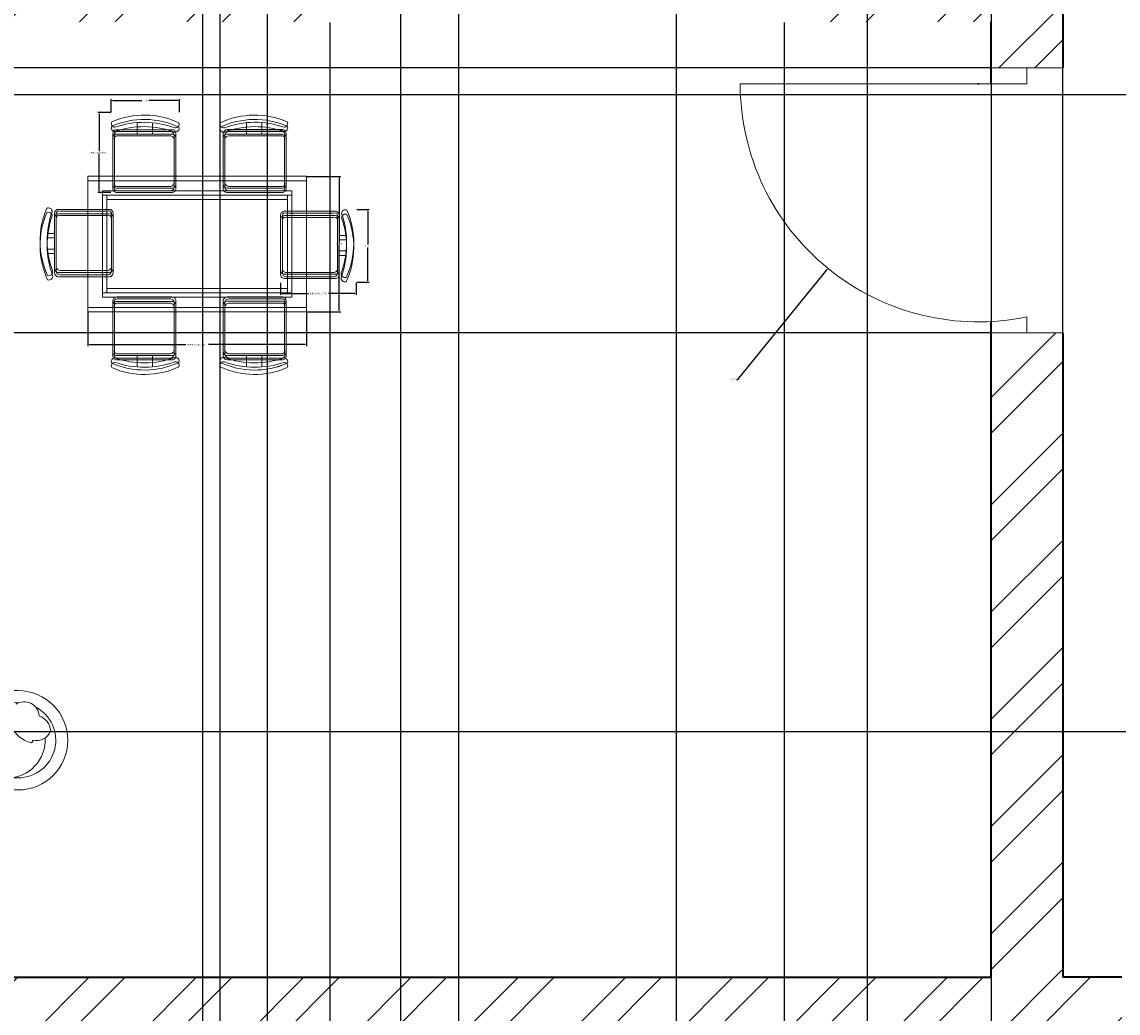
# Model space of a CAD drawing. Units: inches. Extents: x 1748 to 2382, y 1346 to 2284.
# Tile 10 of 26: x 2009 to 2147, y 1730 to 1855. Entities that reach past the tile are written whole.
import ezdxf

# ---------------------------------------------------------------- set-up
doc = ezdxf.new("R2010")
doc.units = ezdxf.units.IN
for name, color, linetype, lineweight in [('A-ANNO-DIMS', 2, 'Continuous', 18), ('A-DOOR', 21, 'Continuous', 18), ('A-FURN', 8, 'Continuous', 13), ('A-WALL', 7, 'Continuous', 35), ('A-WALL-PATT', 9, 'Continuous', 13)]:
    doc.layers.add(name, color=color, linetype=linetype, lineweight=lineweight)
doc.styles.get("Standard").update_dxf_attribs({"font": 'arial.ttf'})
doc.dimstyles.get("Standard").update_dxf_attribs({"dimtxt": 0.18, "dimasz": 0.18, "dimexe": 0.18, "dimexo": 0.0625, "dimgap": 0.09, "dimtad": 0, "dimtih": 1, "dimtoh": 1, "dimdec": 4, "dimzin": 0, "dimdsep": 46, "dimtxsty": 'Standard', "dimcen": 0.09, "dimadec": 0, "dimazin": 0, "dimtfac": 1, "dimtdec": 4, "dimtofl": 0, "dimtmove": 0, "dimatfit": 3, "dimfxl": 1, "dimtolj": 1, "dimtzin": 0, "dimarcsym": 0})

# ---------------------------------------------------------------- blocks, each defined once
blk = doc.blocks.new('TABLE-DINING')
for points in [[(0, 17.02), (27.45, 17.02), (27.45, 0.55), (0, 0.55)], [(0, 17.02), (27.45, 17.02), (27.45, 0.55), (0, 0.55)], [(0, 16.47), (27.45, 16.47), (27.45, 0), (0, 0)], [(0, 16.47), (27.45, 16.47), (27.45, 0), (0, 0)], [(1.83, 15.19), (25.62, 15.19), (25.62, 2.38), (1.83, 2.38)], [(1.83, 15.19), (25.62, 15.19), (25.62, 2.38), (1.83, 2.38)], [(1.83, 14.64), (25.62, 14.64), (25.62, 1.83), (1.83, 1.83)], [(1.83, 14.64), (25.62, 14.64), (25.62, 1.83), (1.83, 1.83)], [(2.38, 14.64), (25.07, 14.64), (25.07, 2.93), (2.38, 2.93)], [(2.38, 14.64), (25.07, 14.64), (25.07, 2.93), (2.38, 2.93)], [(2.38, 14.09), (25.07, 14.09), (25.07, 2.38), (2.38, 2.38)], [(2.38, 14.09), (25.07, 14.09), (25.07, 2.38), (2.38, 2.38)]]:
    blk.add_lwpolyline(points, close=True)
blk = doc.blocks.new('CHAIR-LOUNGE')
blk.add_line((1.52, 6.05), (1.51, 0.29))
at = {"ltscale": 0.03}
blk.add_lwpolyline([(1.51, 0.29, -0.369229), (0, 0.29), (0.01, 6.05, -1), (12.48, 6.04), (12.47, 0.28, -0.369229), (10.96, 0.28)], format="xyb", close=True, dxfattribs=at)
blk.add_lwpolyline([(2.05, 8.23, -0.785087), (10.96, 6.04), (10.96, 0.28)], format="xyb")
for centre, radius, start, end in [((5.21, 8.01), 2.13, 94.9999, 161.3534), ((4.35, 8.32), 1.94, 346.6403, 69.4695), ((3.29, 6.8), 1.89, 92.9922, 214.1401), ((6.24, 4.71), 4.72, 359.9461, 93.658), ((3, 8.54), 3.66, 247.0143, 344.2857), ((6.33, 7.66), 0.226, 330.6238, 113.7423), ((6.24, 6.05), 4.72, 178.8536, 179.9461)]:
    blk.add_arc(centre, radius, start, end)
blk = doc.blocks.new('CHAIR-DINING-SIDE')
for points in [[(0.45, 8.2, -0.175809), (7.92, 8.14, 0.578392), (8.49, 8.77, 0.214524), (0.05, 8.88, 0.552014), (0.45, 8.2, -0.065079)], [(0.45, 8.2, -0.175809), (7.92, 8.14, 0.578392), (8.49, 8.77, 0.214524), (0.05, 8.88, 0.552014), (0.45, 8.2, -0.065079)], [(0.45, 7.65, -0.175809), (7.92, 7.6, 0.578392), (8.49, 8.22, 0.214524), (0.05, 8.33, 0.552014), (0.45, 7.65, -0.065079)], [(0.45, 7.65, -0.175809), (7.92, 7.6, 0.578392), (8.49, 8.22, 0.214524), (0.05, 8.33, 0.552014), (0.45, 7.65, -0.065079)], [(5.17, 7.9), (5.17, 8.78, -0.064759)], [(5.17, 7.9), (5.17, 8.78, -0.064759)], [(7.61, 7.9), (0.67, 7.9, 0.414214), (0.18, 7.42), (0.18, 1.03, 0.414214), (0.67, 0.55), (7.61, 0.55, 0.414214), (8.09, 1.03), (8.09, 7.42, 0.414214), (7.61, 7.9)], [(7.61, 7.9), (0.67, 7.9, 0.414214), (0.18, 7.42), (0.18, 1.03, 0.414214), (0.67, 0.55), (7.61, 0.55, 0.414214), (8.09, 1.03), (8.09, 7.42, 0.414214), (7.61, 7.9)], [(7.61, 7.35), (0.67, 7.35, 0.414214), (0.18, 6.87), (0.18, 0.49, 0.414214), (0.67, 0), (7.61, 0, 0.414214), (8.09, 0.49), (8.09, 6.87, 0.414214), (7.61, 7.35)], [(7.61, 7.35), (0.67, 7.35, 0.414214), (0.18, 6.87), (0.18, 0.49, 0.414214), (0.67, 0), (7.61, 0, 0.414214), (8.09, 0.49), (8.09, 6.87, 0.414214), (7.61, 7.35)], [(5.17, 7.35), (5.17, 8.23, -0.064759)], [(5.17, 7.35), (5.17, 8.23, -0.064759)]]:
    blk.add_lwpolyline(points, format="xyb")
for points in [[(3.23, 8.79), (3.23, 7.9)], [(3.23, 8.79), (3.23, 7.9)], [(3.23, 8.25), (3.23, 7.35)], [(3.23, 8.25), (3.23, 7.35)]]:
    blk.add_lwpolyline(points)
for points in [[(0.67, 7.68), (7.39, 7.68, -0.414214), (7.87, 7.2), (7.87, 1.25, -0.414214), (7.39, 0.77), (0.67, 0.77, -0.512069), (0.4, 1.25), (0.4, 7.2, -0.512069)], [(0.67, 7.68), (7.39, 7.68, -0.414214), (7.87, 7.2), (7.87, 1.25, -0.414214), (7.39, 0.77), (0.67, 0.77, -0.512069), (0.4, 1.25), (0.4, 7.2, -0.512069)], [(0.67, 7.13), (7.39, 7.13, -0.414214), (7.87, 6.65), (7.87, 0.7, -0.414214), (7.39, 0.22), (0.67, 0.22, -0.512069), (0.4, 0.7), (0.4, 6.65, -0.512069)], [(0.67, 7.13), (7.39, 7.13, -0.414214), (7.87, 6.65), (7.87, 0.7, -0.414214), (7.39, 0.22), (0.67, 0.22, -0.512069), (0.4, 0.7), (0.4, 6.65, -0.512069)]]:
    blk.add_lwpolyline(points, format="xyb", close=True)
blk = doc.blocks.new('CHAIR-DINING-END')
for points in [[(7.35, 8.4, 0.414214), (6.87, 8.88), (0.49, 8.88, 0.414214), (0, 8.4), (0, 1.46, 0.414214), (0.49, 0.97), (6.87, 0.97, 0.414214), (7.35, 1.46), (7.35, 8.4)], [(7.35, 8.4, 0.414214), (6.87, 8.88), (0.49, 8.88, 0.414214), (0, 8.4), (0, 1.46, 0.414214), (0.49, 0.97), (6.87, 0.97, 0.414214), (7.35, 1.46), (7.35, 8.4)], [(7.35, 7.85, 0.414214), (6.87, 8.33), (0.49, 8.33, 0.414214), (0, 7.85), (0, 0.91, 0.414214), (0.49, 0.42), (6.87, 0.42, 0.414214), (7.35, 0.91), (7.35, 7.85)], [(7.35, 7.85, 0.414214), (6.87, 8.33), (0.49, 8.33, 0.414214), (0, 7.85), (0, 0.91, 0.414214), (0.49, 0.42), (6.87, 0.42, 0.414214), (7.35, 0.91), (7.35, 7.85)], [(7.65, 8.61, -0.175809), (7.6, 1.14, 0.578392), (8.22, 0.57, 0.214524), (8.33, 9.01, 0.552014), (7.65, 8.61, -0.065079)], [(7.65, 8.61, -0.175809), (7.6, 1.14, 0.578392), (8.22, 0.57, 0.214524), (8.33, 9.01, 0.552014), (7.65, 8.61, -0.065079)], [(7.65, 8.06, -0.175809), (7.6, 0.59, 0.578392), (8.22, 0.02, 0.214524), (8.33, 8.46, 0.552014), (7.65, 8.06, -0.065079)], [(7.65, 8.06, -0.175809), (7.6, 0.59, 0.578392), (8.22, 0.02, 0.214524), (8.33, 8.46, 0.552014), (7.65, 8.06, -0.065079)], [(7.35, 3.89), (8.23, 3.89, -0.064759)], [(7.35, 3.89), (8.23, 3.89, -0.064759)], [(7.35, 3.34), (8.23, 3.34, -0.064759)], [(7.35, 3.34), (8.23, 3.34, -0.064759)]]:
    blk.add_lwpolyline(points, format="xyb")
for points in [[(7.13, 8.39), (7.13, 1.67, -0.414214), (6.65, 1.19), (0.7, 1.19, -0.414214), (0.22, 1.67), (0.22, 8.39, -0.512069), (0.7, 8.66), (6.65, 8.66, -0.512069)], [(7.13, 8.39), (7.13, 1.67, -0.414214), (6.65, 1.19), (0.7, 1.19, -0.414214), (0.22, 1.67), (0.22, 8.39, -0.512069), (0.7, 8.66), (6.65, 8.66, -0.512069)], [(7.13, 7.84), (7.13, 1.13, -0.414214), (6.65, 0.64), (0.7, 0.64, -0.414214), (0.22, 1.13), (0.22, 7.84, -0.512069), (0.7, 8.11), (6.65, 8.11, -0.512069)], [(7.13, 7.84), (7.13, 1.12, -0.414214), (6.65, 0.64), (0.7, 0.64, -0.414214), (0.22, 1.12), (0.22, 7.84, -0.512069), (0.7, 8.11), (6.65, 8.11, -0.512069)]]:
    blk.add_lwpolyline(points, format="xyb", close=True)
for points in [[(8.25, 5.84), (7.35, 5.84)], [(8.25, 5.84), (7.35, 5.84)], [(8.25, 5.29), (7.35, 5.29)], [(8.25, 5.29), (7.35, 5.29)]]:
    blk.add_lwpolyline(points)
blk = doc.blocks.new('*D18')
at = {"layer": 'A-ANNO-DIMS', "color": 0, "lineweight": -2, "transparency": 16777216}
for p, q in [((2017.56, 1818.37), (2017.56, 1814.14)), ((2045, 1818.37), (2045, 1814.14)), ((2017.74, 1814.32), (2029.85, 1814.32)), ((2044.82, 1814.32), (2032.71, 1814.32))]:
    blk.add_line(p, q, dxfattribs=at)
at = {"layer": 'A-ANNO-DIMS', "color": 0, "transparency": 16777216}
for points in [[(2017.74, 1814.35), (2017.74, 1814.29), (2017.56, 1814.32)], [(2044.82, 1814.35), (2044.82, 1814.29), (2045, 1814.32)]]:
    blk.add_solid(points, dxfattribs=at)
at = {"layer": 'Defpoints', "color": 0, "transparency": 16777216}
for p in [(2017.56, 1818.44), (2045, 1818.44), (2045, 1814.32)]:
    blk.add_point(p, dxfattribs=at)
at = {"layer": 'A-ANNO-DIMS', "color": 0, "transparency": 16777216, "insert": (2031.28, 1814.32), "char_height": 0.18, "attachment_point": 5}
blk.add_mtext('\\A1;DINING TABLE 27 TYP.', dxfattribs=at)
blk = doc.blocks.new('*D19')
at = {"layer": 'A-ANNO-DIMS', "color": 0, "lineweight": -2, "transparency": 16777216}
for p, q in [((2045.06, 1835.45), (2049.3, 1835.45)), ((2049.12, 1835.27), (2049.12, 1827.13)), ((2049.12, 1818.62), (2049.12, 1826.77)), ((2045.06, 1818.44), (2049.3, 1818.44))]:
    blk.add_line(p, q, dxfattribs=at)
at = {"layer": 'A-ANNO-DIMS', "color": 0, "transparency": 16777216}
for points in [[(2049.09, 1835.27), (2049.15, 1835.27), (2049.12, 1835.45)], [(2049.09, 1818.62), (2049.15, 1818.62), (2049.12, 1818.44)]]:
    blk.add_solid(points, dxfattribs=at)
at = {"layer": 'Defpoints', "color": 0, "transparency": 16777216}
for p in [(2045, 1835.45), (2049.12, 1835.45), (2045, 1818.44)]:
    blk.add_point(p, dxfattribs=at)
at = {"layer": 'A-ANNO-DIMS', "color": 0, "transparency": 16777216, "insert": (2049.12, 1826.95), "char_height": 0.18, "attachment_point": 5}
blk.add_mtext('\\A1;17 TYP.', dxfattribs=at)
blk = doc.blocks.new('*D20')
at = {"layer": 'A-ANNO-DIMS', "color": 0, "lineweight": -2, "transparency": 16777216}
for p, q in [((2020.42, 1843.47), (2018.79, 1843.47)), ((2018.97, 1843.29), (2018.97, 1838.62)), ((2018.97, 1833.59), (2018.97, 1838.26)), ((2020.42, 1833.41), (2018.79, 1833.41))]:
    blk.add_line(p, q, dxfattribs=at)
at = {"layer": 'A-ANNO-DIMS', "color": 0, "transparency": 16777216}
for points in [[(2018.94, 1843.29), (2019, 1843.29), (2018.97, 1843.47)], [(2018.94, 1833.59), (2019, 1833.59), (2018.97, 1833.41)]]:
    blk.add_solid(points, dxfattribs=at)
at = {"layer": 'Defpoints', "color": 0, "transparency": 16777216}
for p in [(2018.97, 1843.47), (2020.48, 1843.47), (2020.48, 1833.41)]:
    blk.add_point(p, dxfattribs=at)
at = {"layer": 'A-ANNO-DIMS', "color": 0, "transparency": 16777216, "insert": (2018.97, 1838.44), "char_height": 0.18, "attachment_point": 5}
blk.add_mtext('\\A1;SIDE CHAIR 10 TYP.', dxfattribs=at)
blk = doc.blocks.new('*D21')
at = {"layer": 'A-ANNO-DIMS', "color": 0, "lineweight": -2, "transparency": 16777216}
for p, q in [((2020.48, 1843.53), (2020.48, 1845.15)), ((2020.66, 1844.97), (2024.31, 1844.97)), ((2028.87, 1844.97), (2025.22, 1844.97)), ((2029.05, 1843.53), (2029.05, 1845.15))]:
    blk.add_line(p, q, dxfattribs=at)
at = {"layer": 'A-ANNO-DIMS', "color": 0, "transparency": 16777216}
for points in [[(2020.66, 1845), (2020.66, 1844.94), (2020.48, 1844.97)], [(2028.87, 1845), (2028.87, 1844.94), (2029.05, 1844.97)]]:
    blk.add_solid(points, dxfattribs=at)
at = {"layer": 'Defpoints', "color": 0, "transparency": 16777216}
for p in [(2029.05, 1844.97), (2020.48, 1843.47), (2029.05, 1843.47)]:
    blk.add_point(p, dxfattribs=at)
at = {"layer": 'A-ANNO-DIMS', "color": 0, "transparency": 16777216, "insert": (2024.76, 1844.97), "char_height": 0.18, "attachment_point": 5}
blk.add_mtext('\\A1;9 TYP.', dxfattribs=at)
blk = doc.blocks.new('*D22')
at = {"layer": 'A-ANNO-DIMS', "color": 0, "lineweight": -2, "transparency": 16777216}
for p, q in [((2041.76, 1822.09), (2041.76, 1820.55)), ((2051.26, 1822.09), (2051.26, 1820.55)), ((2041.94, 1820.73), (2045.26, 1820.73)), ((2051.08, 1820.73), (2047.76, 1820.73))]:
    blk.add_line(p, q, dxfattribs=at)
at = {"layer": 'A-ANNO-DIMS', "color": 0, "transparency": 16777216}
for points in [[(2041.94, 1820.76), (2041.94, 1820.7), (2041.76, 1820.73)], [(2051.08, 1820.76), (2051.08, 1820.7), (2051.26, 1820.73)]]:
    blk.add_solid(points, dxfattribs=at)
at = {"layer": 'Defpoints', "color": 0, "transparency": 16777216}
for p in [(2041.76, 1822.16), (2051.26, 1822.16), (2051.26, 1820.73)]:
    blk.add_point(p, dxfattribs=at)
at = {"layer": 'A-ANNO-DIMS', "color": 0, "transparency": 16777216, "insert": (2046.51, 1820.73), "char_height": 0.18, "attachment_point": 5}
blk.add_mtext('\\A1;END CHAIR 10 TYP.', dxfattribs=at)
blk = doc.blocks.new('*D23')
at = {"layer": 'A-ANNO-DIMS', "color": 0, "lineweight": -2, "transparency": 16777216}
for p, q in [((2051.32, 1831.27), (2052.87, 1831.27)), ((2052.69, 1831.09), (2052.69, 1826.9)), ((2052.69, 1822.34), (2052.69, 1826.53)), ((2051.32, 1822.16), (2052.87, 1822.16))]:
    blk.add_line(p, q, dxfattribs=at)
at = {"layer": 'A-ANNO-DIMS', "color": 0, "transparency": 16777216}
for points in [[(2052.66, 1831.09), (2052.72, 1831.09), (2052.69, 1831.27)], [(2052.66, 1822.34), (2052.72, 1822.34), (2052.69, 1822.16)]]:
    blk.add_solid(points, dxfattribs=at)
at = {"layer": 'Defpoints', "color": 0, "transparency": 16777216}
for p in [(2051.26, 1831.27), (2052.69, 1831.27), (2051.26, 1822.16)]:
    blk.add_point(p, dxfattribs=at)
at = {"layer": 'A-ANNO-DIMS', "color": 0, "transparency": 16777216, "insert": (2052.69, 1826.71), "char_height": 0.18, "attachment_point": 5}
blk.add_mtext('\\A1;9 TYP.', dxfattribs=at)
blk = doc.blocks.new('*D36')
at = {"layer": 'A-ANNO-DIMS', "color": 0, "lineweight": -2, "transparency": 16777216}
for p, q in [((2031.96, 1970.29), (2031.96, 1360.47)), ((2130.96, 1970.29), (2130.96, 1360.47)), ((2032.14, 1360.65), (2081.24, 1360.65)), ((2130.78, 1360.65), (2081.68, 1360.65))]:
    blk.add_line(p, q, dxfattribs=at)
at = {"layer": 'A-ANNO-DIMS', "color": 0, "transparency": 16777216}
for points in [[(2032.14, 1360.68), (2032.14, 1360.62), (2031.96, 1360.65)], [(2130.78, 1360.68), (2130.78, 1360.62), (2130.96, 1360.65)]]:
    blk.add_solid(points, dxfattribs=at)
at = {"layer": 'Defpoints', "color": 0, "transparency": 16777216}
for p in [(2031.96, 1970.35), (2130.96, 1970.35), (2130.96, 1360.65)]:
    blk.add_point(p, dxfattribs=at)
at = {"layer": 'A-ANNO-DIMS', "color": 0, "transparency": 16777216, "insert": (2081.46, 1360.65), "char_height": 0.18, "attachment_point": 5}
blk.add_mtext('\\A1;99', dxfattribs=at)
blk = doc.blocks.new('*D39')
at = {"layer": 'A-ANNO-DIMS', "color": 0, "lineweight": -2, "transparency": 16777216}
for p, q in [((2139.96, 1734.91), (2139.96, 2274.93)), ((2197.07, 1734.91), (2197.07, 2274.93)), ((2140.14, 2274.75), (2168.14, 2274.75)), ((2196.89, 2274.75), (2168.89, 2274.75))]:
    blk.add_line(p, q, dxfattribs=at)
at = {"layer": 'A-ANNO-DIMS', "color": 0, "transparency": 16777216}
for points in [[(2140.14, 2274.78), (2140.14, 2274.72), (2139.96, 2274.75)], [(2196.89, 2274.78), (2196.89, 2274.72), (2197.07, 2274.75)]]:
    blk.add_solid(points, dxfattribs=at)
at = {"layer": 'Defpoints', "color": 0, "transparency": 16777216}
for p in [(2197.07, 2274.75), (2139.96, 1734.85), (2197.07, 1734.85)]:
    blk.add_point(p, dxfattribs=at)
at = {"layer": 'A-ANNO-DIMS', "color": 0, "transparency": 16777216, "insert": (2168.52, 2274.75), "char_height": 0.18, "attachment_point": 5}
blk.add_mtext('\\A1;57.11', dxfattribs=at)
blk = doc.blocks.new('*D48')
at = {"layer": 'A-ANNO-DIMS', "color": 0, "lineweight": -2, "transparency": 16777216}
for p, q in [((2130.9, 1849.07), (1779.88, 1849.07)), ((1780.06, 1848.89), (1780.06, 1832.62)), ((1780.06, 1815.98), (1780.06, 1832.25)), ((2130.9, 1815.8), (1779.88, 1815.8))]:
    blk.add_line(p, q, dxfattribs=at)
at = {"layer": 'A-ANNO-DIMS', "color": 0, "transparency": 16777216}
for points in [[(1780.03, 1848.89), (1780.09, 1848.89), (1780.06, 1849.07)], [(1780.03, 1815.98), (1780.09, 1815.98), (1780.06, 1815.8)]]:
    blk.add_solid(points, dxfattribs=at)
at = {"layer": 'Defpoints', "color": 0, "transparency": 16777216}
for p in [(1780.06, 1849.07), (2130.96, 1849.07), (2130.96, 1815.8)]:
    blk.add_point(p, dxfattribs=at)
at = {"layer": 'A-ANNO-DIMS', "color": 0, "transparency": 16777216, "insert": (1780.06, 1832.43), "char_height": 0.18, "attachment_point": 5}
blk.add_mtext('\\A1;33.27', dxfattribs=at)
blk = doc.blocks.new('*D51')
at = {"layer": 'A-ANNO-DIMS', "color": 0, "lineweight": -2, "transparency": 16777216}
for p, q in [((1968.44, 2223.79), (1968.44, 1360.47)), ((2040.07, 2223.79), (2040.07, 1360.47)), ((1968.62, 1360.65), (2003.86, 1360.65)), ((2039.89, 1360.65), (2004.65, 1360.65))]:
    blk.add_line(p, q, dxfattribs=at)
at = {"layer": 'A-ANNO-DIMS', "color": 0, "transparency": 16777216}
for points in [[(1968.62, 1360.68), (1968.62, 1360.62), (1968.44, 1360.65)], [(2039.89, 1360.68), (2039.89, 1360.62), (2040.07, 1360.65)]]:
    blk.add_solid(points, dxfattribs=at)
at = {"layer": 'Defpoints', "color": 0, "transparency": 16777216}
for p in [(1968.44, 2223.85), (2040.07, 2223.85), (2040.07, 1360.65)]:
    blk.add_point(p, dxfattribs=at)
at = {"layer": 'A-ANNO-DIMS', "color": 0, "transparency": 16777216, "insert": (2004.26, 1360.65), "char_height": 0.18, "attachment_point": 5}
blk.add_mtext('\\A1;71.62', dxfattribs=at)
blk = doc.blocks.new('*D52')
at = {"layer": 'A-ANNO-DIMS', "color": 0, "lineweight": -2, "transparency": 16777216}
for p, q in [((2064.07, 2223.79), (2064.07, 1360.47)), ((2091.4, 2223.79), (2091.4, 1360.47)), ((2064.25, 1360.65), (2077.34, 1360.65)), ((2091.22, 1360.65), (2078.13, 1360.65))]:
    blk.add_line(p, q, dxfattribs=at)
at = {"layer": 'A-ANNO-DIMS', "color": 0, "transparency": 16777216}
for points in [[(2064.25, 1360.68), (2064.25, 1360.62), (2064.07, 1360.65)], [(2091.22, 1360.68), (2091.22, 1360.62), (2091.4, 1360.65)]]:
    blk.add_solid(points, dxfattribs=at)
at = {"layer": 'Defpoints', "color": 0, "transparency": 16777216}
for p in [(2064.07, 2223.85), (2091.4, 2223.85), (2091.4, 1360.65)]:
    blk.add_point(p, dxfattribs=at)
at = {"layer": 'A-ANNO-DIMS', "color": 0, "transparency": 16777216, "insert": (2077.73, 1360.65), "char_height": 0.18, "attachment_point": 5}
blk.add_mtext('\\A1;27.33', dxfattribs=at)
blk = doc.blocks.new('*D53')
at = {"layer": 'A-ANNO-DIMS', "color": 0, "lineweight": -2, "transparency": 16777216}
for p, q in [((2115.4, 2223.79), (2115.4, 1360.47)), ((2167.02, 2223.79), (2167.02, 1360.47)), ((2115.58, 1360.65), (2140.81, 1360.65)), ((2166.84, 1360.65), (2141.6, 1360.65))]:
    blk.add_line(p, q, dxfattribs=at)
at = {"layer": 'A-ANNO-DIMS', "color": 0, "transparency": 16777216}
for points in [[(2115.58, 1360.68), (2115.58, 1360.62), (2115.4, 1360.65)], [(2166.84, 1360.68), (2166.84, 1360.62), (2167.02, 1360.65)]]:
    blk.add_solid(points, dxfattribs=at)
at = {"layer": 'Defpoints', "color": 0, "transparency": 16777216}
for p in [(2115.4, 2223.85), (2167.02, 2223.85), (2167.02, 1360.65)]:
    blk.add_point(p, dxfattribs=at)
at = {"layer": 'A-ANNO-DIMS', "color": 0, "transparency": 16777216, "insert": (2141.21, 1360.65), "char_height": 0.18, "attachment_point": 5}
blk.add_mtext('\\A1;51.62', dxfattribs=at)
blk = doc.blocks.new('*D60')
at = {"layer": 'A-ANNO-DIMS', "color": 0, "lineweight": -2, "transparency": 16777216}
for p, q in [((2206.01, 1845.68), (1779.88, 1845.68)), ((1780.06, 1845.5), (1780.06, 1805.86)), ((1780.06, 1765.86), (1780.06, 1805.5)), ((2206.01, 1765.68), (1779.88, 1765.68))]:
    blk.add_line(p, q, dxfattribs=at)
at = {"layer": 'A-ANNO-DIMS', "color": 0, "transparency": 16777216}
for points in [[(1780.03, 1845.5), (1780.09, 1845.5), (1780.06, 1845.68)], [(1780.03, 1765.86), (1780.09, 1765.86), (1780.06, 1765.68)]]:
    blk.add_solid(points, dxfattribs=at)
at = {"layer": 'Defpoints', "color": 0, "transparency": 16777216}
for p in [(1780.06, 1845.68), (2206.07, 1845.68), (2206.07, 1765.68)]:
    blk.add_point(p, dxfattribs=at)
at = {"layer": 'A-ANNO-DIMS', "color": 0, "transparency": 16777216, "insert": (1780.06, 1805.68), "char_height": 0.18, "attachment_point": 5}
blk.add_mtext('\\A1;80', dxfattribs=at)
blk = doc.blocks.new('*D61')
at = {"layer": 'A-ANNO-DIMS', "color": 0, "lineweight": -2, "transparency": 16777216}
for p, q in [((2047.92, 1854.79), (2047.92, 1360.47)), ((2104.96, 1854.79), (2104.96, 1360.47)), ((2048.1, 1360.65), (2076.04, 1360.65)), ((2104.78, 1360.65), (2076.83, 1360.65))]:
    blk.add_line(p, q, dxfattribs=at)
at = {"layer": 'A-ANNO-DIMS', "color": 0, "transparency": 16777216}
for points in [[(2048.1, 1360.68), (2048.1, 1360.62), (2047.92, 1360.65)], [(2104.78, 1360.68), (2104.78, 1360.62), (2104.96, 1360.65)]]:
    blk.add_solid(points, dxfattribs=at)
at = {"layer": 'Defpoints', "color": 0, "transparency": 16777216}
for p in [(2047.92, 1854.85), (2104.96, 1854.85), (2104.96, 1360.65)]:
    blk.add_point(p, dxfattribs=at)
at = {"layer": 'A-ANNO-DIMS', "color": 0, "transparency": 16777216, "insert": (2076.44, 1360.65), "char_height": 0.18, "attachment_point": 5}
blk.add_mtext('\\A1;57.04', dxfattribs=at)
blk = doc.blocks.new('*D78')
at = {"layer": 'A-ANNO-DIMS', "color": 0, "lineweight": -2, "transparency": 16777216}
for p, q in [((2034.13, 2132.54), (2034.13, 1360.47)), ((2056.8, 2127.06), (2056.8, 1360.47)), ((2034.31, 1360.65), (2045, 1360.65)), ((2056.62, 1360.65), (2045.93, 1360.65))]:
    blk.add_line(p, q, dxfattribs=at)
at = {"layer": 'A-ANNO-DIMS', "color": 0, "transparency": 16777216}
for points in [[(2034.31, 1360.68), (2034.31, 1360.62), (2034.13, 1360.65)], [(2056.62, 1360.68), (2056.62, 1360.62), (2056.8, 1360.65)]]:
    blk.add_solid(points, dxfattribs=at)
at = {"layer": 'Defpoints', "color": 0, "transparency": 16777216}
for p in [(2034.13, 2132.6), (2056.8, 2127.13), (2056.8, 1360.65)]:
    blk.add_point(p, dxfattribs=at)
at = {"layer": 'A-ANNO-DIMS', "color": 0, "transparency": 16777216, "insert": (2045.47, 1360.65), "char_height": 0.18, "attachment_point": 5}
blk.add_mtext('\\A1;22.663', dxfattribs=at)
blk = doc.blocks.new('*D82')
at = {"layer": 'A-ANNO-DIMS', "color": 0, "lineweight": -2, "transparency": 16777216}
for p, q in [((2129.27, 1847.07), (2129.45, 1847.07)), ((2129.36, 1846.98), (2129.36, 1847.16)), ((2099.18, 1809.95), (2110.38, 1823.73)), ((2099, 1809.95), (2099.18, 1809.95))]:
    blk.add_line(p, q, dxfattribs=at)
at = {"layer": 'A-ANNO-DIMS', "color": 0, "transparency": 16777216}
blk.add_solid([(2110.36, 1823.75), (2110.41, 1823.71), (2110.5, 1823.87)], dxfattribs=at)
at = {"layer": 'Defpoints', "color": 0, "transparency": 16777216}
for p in [(2129.36, 1847.07), (2110.5, 1823.87)]:
    blk.add_point(p, dxfattribs=at)
at = {"layer": 'A-ANNO-DIMS', "color": 0, "transparency": 16777216, "insert": (2098.59, 1809.95), "char_height": 0.18, "attachment_point": 5}
blk.add_mtext('\\A1;R29.9', dxfattribs=at)

msp = doc.modelspace()

# ---------------------------------------------------------------- hatches: boundary and pattern name
at = {"layer": 'A-WALL-PATT'}
h = msp.add_hatch(dxfattribs=at)
h.set_pattern_fill('ANSI32', color=256)
h.paths.add_polyline_path([(1900.6426, 1652.723), (1896.1426, 1652.723), (1896.1426, 1629.9029), (1900.6426, 1629.9029)])
h.paths.add_polyline_path([(2206.0699, 1859.3497), (2197.0699, 1859.3497), (2197.0699, 1734.8497), (2206.0699, 1734.8497)], flags=17)
h.paths.add_polyline_path([(2297.4607, 1865.3269), (2288.4607, 1865.3269), (2288.4607, 1734.8497), (2206.0699, 1734.8497), (2180.4551, 1734.8497), (2180.4551, 1725.8497), (2197.0699, 1725.8497), (2206.0699, 1725.8497), (2288.4607, 1725.8497), (2288.4607, 1705.3038), (2297.4607, 1705.3038)])
h.paths.add_polyline_path([(2139.9607, 1815.8001), (2135.4607, 1815.8001), (2130.9607, 1815.8001), (2130.9607, 1734.8497), (1900.6426, 1734.8497), (1900.6426, 1738.9477), (1898.3926, 1738.9477), (1896.1426, 1738.9477), (1896.1426, 1734.8497), (1857.1426, 1734.8497), (1857.1426, 1725.8497), (1896.1426, 1725.8497), (1896.1426, 1712.723), (1900.6426, 1712.723), (1900.6426, 1725.8497), (2006.4607, 1725.8497), (2006.4607, 1637.448), (2010.9607, 1637.448), (2010.9607, 1725.8497), (2139.9607, 1725.8497), (2147.389, 1725.8497), (2147.389, 1730.3497), (2147.389, 1734.8497), (2139.9607, 1734.8497)])
h.paths.add_polyline_path([(2149.8497, 1917.8497), (2149.8497, 1922.3497), (2139.9607, 1922.3497), (2139.9607, 1979.3497), (2030.4607, 1979.3497), (2030.4607, 2069.8971), (2028.2107, 2069.8971), (2025.9607, 2069.8971), (2025.9607, 1979.3497), (1869.9607, 1979.3497), (1869.9607, 1998.93), (1865.4607, 1998.93), (1865.4607, 1979.3497), (1821.9607, 1979.3497), (1821.9607, 1952.7922), (1826.9306, 1952.7922), (1830.9607, 1952.7922), (1830.9607, 1970.3497), (1962.9607, 1970.3497), (1962.9607, 1926.5713), (1967.4607, 1926.5713), (1967.4607, 1970.3497), (2027.4607, 1970.3497), (2027.4607, 1898.3497), (2004.9604, 1898.3497), (2004.9604, 1893.8497), (2027.4607, 1893.8497), (2027.4607, 1859.3497), (1958.8973, 1859.3497), (1958.8973, 1854.8497), (2047.917, 1854.8497), (2047.917, 1859.3497), (2031.9607, 1859.3497), (2031.9607, 1970.3497), (2130.9607, 1970.3497), (2130.9607, 1859.3497), (2104.9565, 1859.3497), (2104.9565, 1854.8497), (2130.9607, 1854.8497), (2130.9607, 1849.0684), (2139.9607, 1849.0684), (2139.9607, 1913.3497), (2149.8497, 1913.3497)])
h.paths.add_polyline_path([(1928.9996, 1859.3497), (1830.9607, 1859.3497), (1830.9607, 1892.7922), (1821.9607, 1892.7922), (1821.9607, 1854.8497), (1896.1426, 1854.8497), (1896.1426, 1836.6443), (1898.378, 1836.6443), (1900.6426, 1836.6443), (1900.6426, 1854.8497), (1928.9996, 1854.8497), (1928.9996, 1857.0997)])
h.paths.add_polyline_path([(1980.9604, 1896.0997), (1980.9604, 1898.3497), (1967.4607, 1898.3497), (1967.4607, 1902.3846), (1962.9607, 1902.3846), (1962.9607, 1859.3497), (1967.4607, 1859.3497), (1967.4607, 1893.8497), (1980.9604, 1893.8497)], flags=17)
h.paths.add_polyline_path([(1900.6426, 1776.6443), (1896.1426, 1776.6443), (1896.1426, 1758.0891), (1900.6426, 1758.0891)], flags=17)
h.paths.add_polyline_path([(2297.4607, 2017.2008), (2288.4607, 2017.2008), (2288.4607, 1979.3497), (2213.4607, 1979.3497), (2213.4607, 1922.3497), (2183.3516, 1922.3497), (2183.3516, 1913.3497), (2213.4607, 1913.3497), (2236.234, 1913.3497), (2236.234, 1922.3497), (2222.4607, 1922.3497), (2222.4607, 1931.3497), (2222.4607, 1970.3497), (2288.4607, 1970.3497), (2288.4607, 1922.3497), (2272.1921, 1922.3497), (2272.1921, 1913.3497), (2288.4607, 1913.3497), (2288.4607, 1901.3269), (2297.4607, 1901.3269)])

# ---------------------------------------------------------------- linework, layer by layer
at = {"layer": 'A-DOOR'}
for p, q in [((2130.9607, 1849.0684), (2139.9607, 1849.0684)), ((2139.9607, 1849.0684), (2135.4607, 1849.0684)), ((2135.4607, 1849.0684), (2135.4607, 1847.0684)), ((2135.4607, 1847.0684), (2099.4607, 1847.0684)), ((2135.4607, 1815.8001), (2135.4607, 1817.8001)), ((2130.9607, 1815.8001), (2139.9607, 1815.8001)), ((2139.9607, 1815.8001), (2135.4607, 1815.8001))]:
    msp.add_line(p, q, dxfattribs=at)
msp.add_arc((2129.3584, 1847.0684), 29.8978, 180, 281.77705, dxfattribs=at)
at = {"layer": 'A-FURN'}
for points in [[(2034.7201, 1841.5584, -0.57839206), (2034.1537, 1842.1811, -0.21452438), (2042.5919, 1842.2943, -0.55201397), (2042.1955, 1841.615, 0.1758092), (2034.7201, 1841.5584)], [(2034.7201, 1841.5581, -0.57839206), (2034.1537, 1842.1808, -0.21452438), (2042.5919, 1842.294, -0.55201397), (2042.1955, 1841.6147, 0.1758092), (2034.7201, 1841.5581)], [(2034.7201, 1841.0094, -0.57839206), (2034.1537, 1841.6322, -0.21452438), (2042.5919, 1841.7454, -0.55201397), (2042.1955, 1841.0661, 0.1758092), (2034.7201, 1841.0094)], [(2034.7201, 1841.0092, -0.57839206), (2034.1537, 1841.6319, -0.21452438), (2042.5919, 1841.7451, -0.55201397), (2042.1955, 1841.0658, 0.1758092), (2034.7201, 1841.0092)], [(2037.4749, 1841.3149), (2037.4749, 1842.1926, 0.06475861)], [(2037.4749, 1841.3146), (2037.4749, 1842.1923, 0.06475861)], [(2037.4749, 1840.766), (2037.4749, 1841.6437, 0.06475861)], [(2037.4749, 1840.7657), (2037.4749, 1841.6434, 0.06475861)], [(2041.9771, 1841.3149, -0.41421356), (2042.4627, 1840.8294), (2042.4627, 1834.4483, -0.41421356), (2041.9771, 1833.9627), (2035.0372, 1833.9627, -0.41421356), (2034.5517, 1834.4483), (2034.5517, 1840.8294, -0.41421356), (2035.0372, 1841.3149), (2041.9771, 1841.3149)], [(2041.9772, 1841.3146, -0.41421356), (2042.4627, 1840.8291), (2042.4627, 1834.448, -0.41421356), (2041.9772, 1833.9625), (2035.0372, 1833.9625, -0.41421356), (2034.5517, 1834.448), (2034.5517, 1840.8291, -0.41421356), (2035.0372, 1841.3146), (2041.9772, 1841.3146)], [(2041.9771, 1840.766, -0.41421356), (2042.4627, 1840.2805), (2042.4627, 1833.8994, -0.41421356), (2041.9771, 1833.4138), (2035.0372, 1833.4138, -0.41421356), (2034.5517, 1833.8994), (2034.5517, 1840.2805, -0.41421356), (2035.0372, 1840.766), (2041.9771, 1840.766)], [(2041.9772, 1840.7657, -0.41421356), (2042.4627, 1840.2802), (2042.4627, 1833.8991, -0.41421356), (2041.9772, 1833.4135), (2035.0372, 1833.4135, -0.41421356), (2034.5517, 1833.8991), (2034.5517, 1840.2802, -0.41421356), (2035.0372, 1840.7657), (2041.9772, 1840.7657)], [(2013.1305, 1823.5629, -0.57839206), (2012.5078, 1822.9966, -0.21452438), (2012.3946, 1831.4348, -0.55201397), (2013.0739, 1831.0384, 0.17580937), (2013.1305, 1823.5629)], [(2013.1305, 1823.5626, -0.57839206), (2012.5078, 1822.9963, -0.21452438), (2012.3946, 1831.4345, -0.55201397), (2013.0739, 1831.0381, 0.17580937), (2013.1305, 1823.5626)], [(2013.1305, 1823.014, -0.57839206), (2012.5078, 1822.4477, -0.21452438), (2012.3946, 1830.8859, -0.55201397), (2013.0739, 1830.4894, 0.17580937), (2013.1305, 1823.014)], [(2013.1305, 1823.0137, -0.57839206), (2012.5078, 1822.4474, -0.21452438), (2012.3946, 1830.8856, -0.55201397), (2013.0739, 1830.4892, 0.17580937), (2013.1305, 1823.0137)], [(2013.3739, 1830.82, -0.41421356), (2013.8595, 1831.3055), (2020.2406, 1831.3055, -0.41421356), (2020.7261, 1830.82), (2020.7261, 1823.8801, -0.41421356), (2020.2406, 1823.3945), (2013.8595, 1823.3945, -0.41421356), (2013.3739, 1823.8801), (2013.3739, 1830.82)], [(2013.3739, 1830.2711, -0.41421356), (2013.8595, 1830.7566), (2020.2406, 1830.7566, -0.41421356), (2020.7261, 1830.2711), (2020.7261, 1823.3312, -0.41421356), (2020.2406, 1822.8456), (2013.8595, 1822.8456, -0.41421356), (2013.3739, 1823.3312), (2013.3739, 1830.2711)], [(2013.374, 1830.8197, -0.41421356), (2013.8595, 1831.3052), (2020.2406, 1831.3052, -0.41421356), (2020.7261, 1830.8197), (2020.7261, 1823.8798, -0.41421356), (2020.2406, 1823.3943), (2013.8595, 1823.3943, -0.41421356), (2013.374, 1823.8798), (2013.374, 1830.8197)], [(2013.374, 1830.2708, -0.41421356), (2013.8595, 1830.7563), (2020.2406, 1830.7563, -0.41421356), (2020.7261, 1830.2708), (2020.7261, 1823.3309, -0.41421356), (2020.2406, 1822.8453), (2013.8595, 1822.8453, -0.41421356), (2013.374, 1823.3309), (2013.374, 1830.2708)], [(2013.3739, 1826.3177), (2012.4962, 1826.3177, 0.06475861)], [(2013.374, 1826.3174), (2012.4963, 1826.3174, 0.06475861)], [(2013.3739, 1825.7688), (2012.4962, 1825.7688, 0.06475861)], [(2013.374, 1825.7685), (2012.4963, 1825.7685, 0.06475861)], [(2041.9771, 1812.9492, 0.41421356), (2042.4627, 1813.4347), (2042.4627, 1819.8159, 0.41421356), (2041.9771, 1820.3014), (2035.0372, 1820.3014, 0.41421356), (2034.5517, 1819.8159), (2034.5517, 1813.4347, 0.41421356), (2035.0372, 1812.9492), (2041.9771, 1812.9492)], [(2041.9772, 1812.9489, 0.41421356), (2042.4627, 1813.4344), (2042.4627, 1819.8156, 0.41421356), (2041.9772, 1820.3011), (2035.0372, 1820.3011, 0.41421356), (2034.5517, 1819.8156), (2034.5517, 1813.4344, 0.41421356), (2035.0372, 1812.9489), (2041.9772, 1812.9489)], [(2041.9771, 1812.4003, 0.41421356), (2042.4627, 1812.8858), (2042.4627, 1819.2669, 0.41421356), (2041.9771, 1819.7525), (2035.0372, 1819.7525, 0.41421356), (2034.5517, 1819.2669), (2034.5517, 1812.8858, 0.41421356), (2035.0372, 1812.4003), (2041.9771, 1812.4003)], [(2041.9772, 1812.4, 0.41421356), (2042.4627, 1812.8855), (2042.4627, 1819.2667, 0.41421356), (2041.9772, 1819.7522), (2035.0372, 1819.7522, 0.41421356), (2034.5517, 1819.2667), (2034.5517, 1812.8855, 0.41421356), (2035.0372, 1812.4), (2041.9772, 1812.4)], [(2042.1955, 1812.6492, -0.17580928), (2034.7201, 1812.7058, 0.57839206), (2034.1537, 1812.0831, 0.21452438), (2042.5919, 1811.9698, 0.55201397), (2042.1955, 1812.6492, -0.06507904)], [(2042.1955, 1812.6489, -0.17580928), (2034.7201, 1812.7055, 0.57839206), (2034.1537, 1812.0828, 0.21452438), (2042.5919, 1811.9695, 0.55201397), (2042.1955, 1812.6489, -0.06507904)], [(2037.4749, 1812.9492), (2037.4749, 1812.0715, -0.06475861)], [(2037.4749, 1812.9489), (2037.4749, 1812.0712, -0.06475861)], [(2042.1955, 1812.1002, -0.17580928), (2034.7201, 1812.1569, 0.57839206), (2034.1537, 1811.5341, 0.21452438), (2042.5919, 1811.4209, 0.55201397), (2042.1955, 1812.1002, -0.06507904)], [(2042.1955, 1812.1, -0.17580928), (2034.7201, 1812.1566, 0.57839206), (2034.1537, 1811.5339, 0.21452438), (2042.5919, 1811.4206, 0.55201397), (2042.1955, 1812.1, -0.06507904)], [(2037.4749, 1812.4003), (2037.4749, 1811.5226, -0.06475861)], [(2037.4749, 1812.4), (2037.4749, 1811.5223, -0.06475861)]]:
    msp.add_lwpolyline(points, format="xyb", dxfattribs=at)
for points in [[(2039.4175, 1842.2086), (2039.4175, 1841.3149)], [(2039.4175, 1842.2083), (2039.4175, 1841.3146)], [(2039.4175, 1841.6597), (2039.4175, 1840.766)], [(2039.4175, 1841.6594), (2039.4175, 1840.7657)], [(2012.4803, 1828.2603), (2013.3739, 1828.2603)], [(2012.4803, 1828.26), (2013.374, 1828.26)], [(2012.4803, 1827.7114), (2013.3739, 1827.7114)], [(2012.4803, 1827.7111), (2013.374, 1827.7111)], [(2039.4175, 1812.0555), (2039.4175, 1812.9492)], [(2039.4175, 1812.0553), (2039.4175, 1812.9489)], [(2039.4175, 1811.5066), (2039.4175, 1812.4003)], [(2039.4175, 1811.5063), (2039.4175, 1812.4)]]:
    msp.add_lwpolyline(points, dxfattribs=at)
for points in [[(2041.9742, 1841.0962), (2035.2559, 1841.0962, 0.41421356), (2034.7704, 1840.6107), (2034.7704, 1834.667, 0.41421356), (2035.2559, 1834.1815), (2041.9742, 1834.1815, 0.51206948), (2042.2439, 1834.667), (2042.2439, 1840.6107, 0.51206948)], [(2041.9742, 1841.0959), (2035.2559, 1841.0959, 0.41421356), (2034.7704, 1840.6104), (2034.7704, 1834.6667, 0.41421356), (2035.2559, 1834.1812), (2041.9742, 1834.1812, 0.51206948), (2042.244, 1834.6667), (2042.244, 1840.6104, 0.51206948)], [(2041.9742, 1840.5473), (2035.2559, 1840.5473, 0.41421356), (2034.7704, 1840.0618), (2034.7704, 1834.1181, 0.41421356), (2035.2559, 1833.6326), (2041.9742, 1833.6326, 0.51206948), (2042.2439, 1834.1181), (2042.2439, 1840.0618, 0.51206948)], [(2041.9742, 1840.547), (2035.2559, 1840.547, 0.41421356), (2034.7704, 1840.0615), (2034.7704, 1834.1178, 0.41421356), (2035.2559, 1833.6323), (2041.9742, 1833.6323, 0.51206948), (2042.244, 1834.1178), (2042.244, 1840.0615, 0.51206948)], [(2013.5927, 1830.8171), (2013.5927, 1824.0988, 0.41421356), (2014.0782, 1823.6133), (2020.0219, 1823.6133, 0.41421356), (2020.5074, 1824.0988), (2020.5074, 1830.8171, 0.51206948), (2020.0219, 1831.0868), (2014.0782, 1831.0868, 0.51206948)], [(2013.5927, 1830.8168), (2013.5927, 1824.0985, 0.41421356), (2014.0782, 1823.613), (2020.0219, 1823.613, 0.41421356), (2020.5074, 1824.0985), (2020.5074, 1830.8168, 0.51206948), (2020.0219, 1831.0865), (2014.0782, 1831.0865, 0.51206948)], [(2013.5927, 1830.2682), (2013.5927, 1823.5499, 0.41421356), (2014.0782, 1823.0644), (2020.0219, 1823.0644, 0.41421356), (2020.5074, 1823.5499), (2020.5074, 1830.2682, 0.51206948), (2020.0219, 1830.5379), (2014.0782, 1830.5379, 0.51206948)], [(2013.5927, 1830.2679), (2013.5927, 1823.5496, 0.41421356), (2014.0782, 1823.0641), (2020.0219, 1823.0641, 0.41421356), (2020.5074, 1823.5496), (2020.5074, 1830.2679, 0.51206948), (2020.0219, 1830.5376), (2014.0782, 1830.5376, 0.51206948)], [(2041.9742, 1813.1679), (2035.2559, 1813.1679, -0.41421356), (2034.7704, 1813.6534), (2034.7704, 1819.5971, -0.41421356), (2035.2559, 1820.0827), (2041.9742, 1820.0827, -0.51206948), (2042.2439, 1819.5971), (2042.2439, 1813.6534, -0.51206948)], [(2041.9742, 1813.1676), (2035.2559, 1813.1676, -0.41421356), (2034.7704, 1813.6532), (2034.7704, 1819.5968, -0.41421356), (2035.2559, 1820.0824), (2041.9742, 1820.0824, -0.51206948), (2042.244, 1819.5968), (2042.244, 1813.6532, -0.51206948)], [(2041.9742, 1812.619), (2035.2559, 1812.619, -0.41421356), (2034.7704, 1813.1045), (2034.7704, 1819.0482, -0.41421356), (2035.2559, 1819.5337), (2041.9742, 1819.5337, -0.51206948), (2042.2439, 1819.0482), (2042.2439, 1813.1045, -0.51206948)], [(2041.9742, 1812.6187), (2035.2559, 1812.6187, -0.41421356), (2034.7704, 1813.1042), (2034.7704, 1819.0479, -0.41421356), (2035.2559, 1819.5335), (2041.9742, 1819.5335, -0.51206948), (2042.244, 1819.0479), (2042.244, 1813.1042, -0.51206948)]]:
    msp.add_lwpolyline(points, format="xyb", close=True, dxfattribs=at)
at = {"layer": 'A-WALL'}
for p, q in [((2139.9607, 1913.3497), (2139.9607, 1849.0684)), ((2130.9607, 1847.0684), (2130.9607, 1854.8497)), ((2130.9607, 1734.8497), (2130.9607, 1817.2137)), ((2139.9607, 1815.8001), (2139.9607, 1734.8497)), ((1900.6426, 1734.8497), (2130.9607, 1734.8497)), ((2147.389, 1734.8497), (2139.9607, 1734.8497))]:
    msp.add_line(p, q, dxfattribs=at)

# ---------------------------------------------------------------- block references
at = {"layer": 'A-FURN'}
for name, p in [('CHAIR-DINING-SIDE', (2020.5018, 1833.414)), ('TABLE-DINING', (2017.557, 1818.437)), ('CHAIR-DINING-END', (2041.759, 1822.187))]:
    msp.add_blockref(name, p, dxfattribs=at)
at = {"layer": 'A-FURN', "extrusion": (0, 0, -1), "zscale": -1, "rotation": 180}
msp.add_blockref('CHAIR-DINING-SIDE', (-2020.5018, 1820.3009), dxfattribs=at)
at = {"layer": 'A-FURN', "rotation": 270}
msp.add_blockref('CHAIR-LOUNGE', (2002.7577, 1770.8585), dxfattribs=at)

# ---------------------------------------------------------------- dimensions: what is measured, and where the dimension line sits
at = {"layer": 'A-ANNO-DIMS'}
for base, p1, p2, override, picture, middle in [((2197.0699, 2274.7497), (2139.9607, 1734.8497), (2197.0699, 1734.8497), {"dimdec": 2, "dimlfac": 1, "dimrnd": 0, "dimzin": 0, "dimdsep": 46, "dimlunit": 2}, '*D39', (2168.5153, 2274.7497)), ((2040.0683, 1360.6451), (1968.4445, 2223.8497), (2040.0683, 2223.8497), {"dimdec": 2, "dimlfac": 1, "dimrnd": 0, "dimzin": 0, "dimdsep": 46, "dimlunit": 2}, '*D51', (2004.2564, 1360.6451)), ((2091.3969, 1360.6451), (2064.0683, 2223.8497), (2091.3969, 2223.8497), {"dimdec": 2, "dimlfac": 1, "dimrnd": 0, "dimzin": 0, "dimdsep": 46, "dimlunit": 2}, '*D52', (2077.7326, 1360.6451)), ((2167.0164, 1360.6451), (2115.3969, 2223.8497), (2167.0164, 2223.8497), {"dimdec": 2, "dimlfac": 1, "dimrnd": 0, "dimzin": 0, "dimdsep": 46, "dimlunit": 2}, '*D53', (2141.2066, 1360.6451)), ((2056.7974, 1360.6451), (2034.1341, 2132.5997), (2056.7974, 2127.1257), {"dimdec": 3, "dimlfac": 1, "dimrnd": 0, "dimzin": 0, "dimdsep": 46, "dimlunit": 2}, '*D78', (2045.4658, 1360.6451)), ((2130.9607, 1360.6451), (2031.9607, 1970.3497), (2130.9607, 1970.3497), {"dimdec": 0, "dimlfac": 1, "dimrnd": 0, "dimzin": 0, "dimdsep": 46, "dimlunit": 2}, '*D36', (2081.4607, 1360.6451)), ((2104.9565, 1360.6451), (2047.917, 1854.8497), (2104.9565, 1854.8497), {"dimdec": 2, "dimlfac": 1, "dimrnd": 0, "dimzin": 0, "dimdsep": 46, "dimlunit": 2}, '*D61', (2076.4368, 1360.6451))]:
    dim = msp.add_linear_dim(base=base, p1=p1, p2=p2, dimstyle='Standard', override=override, dxfattribs=at)
    dim.commit()
    dim.dimension.update_dxf_attribs({"geometry": picture, "text_midpoint": middle})
for base, p1, p2, override, picture, middle in [((1780.0607, 1849.0684), (2130.9607, 1815.8001), (2130.9607, 1849.0684), {"dimdec": 2, "dimlfac": 1, "dimrnd": 0, "dimzin": 0, "dimdsep": 46, "dimlunit": 2}, '*D48', (1780.0607, 1832.4343)), ((1780.0607, 1845.6799), (2206.0699, 1765.6799), (2206.0699, 1845.6799), {"dimdec": 0, "dimlfac": 1, "dimrnd": 0, "dimzin": 0, "dimdsep": 46, "dimlunit": 2}, '*D60', (1780.0607, 1805.6799))]:
    dim = msp.add_linear_dim(base=base, p1=p1, p2=p2, angle=90, dimstyle='Standard', override=override, dxfattribs=at)
    dim.commit()
    dim.dimension.update_dxf_attribs({"geometry": picture, "text_midpoint": middle})
dim = msp.add_radius_dim(center=(2129.3584, 1847.0684), mpoint=(2110.4981, 1823.8701), dimstyle='Standard', override={"dimdec": 1, "dimlfac": 1, "dimrnd": 0, "dimzin": 0, "dimdsep": 46, "dimlunit": 2}, dxfattribs=at)
dim.commit()
dim.dimension.update_dxf_attribs({"geometry": '*D82', "text_midpoint": (2098.5918, 1809.9511), "dimtype": 164})
for base, p1, p2, text, picture, middle in [((2029.0462, 1844.9728), (2020.481, 1843.4651), (2029.0462, 1843.4651), '<> TYP.', '*D21', (2024.7636, 1844.9728)), ((2051.2616, 1820.7312), (2041.7592, 1822.1566), (2051.2616, 1822.1566), 'END CHAIR <> TYP.', '*D22', (2046.5104, 1820.7312)), ((2045.0023, 1814.3205), (2017.5565, 1818.4373), (2045.0023, 1818.4373), 'DINING TABLE <> TYP.', '*D18', (2031.2794, 1814.3205))]:
    dim = msp.add_linear_dim(base=base, p1=p1, p2=p2, text=text, dimstyle='Standard', override={"dimdec": 0, "dimlfac": 1, "dimrnd": 0, "dimzin": 0, "dimdsep": 46, "dimlunit": 2}, dxfattribs=at)
    dim.commit()
    dim.dimension.update_dxf_attribs({"geometry": picture, "text_midpoint": middle})
for base, p1, p2, text, picture, middle in [((2018.9733, 1843.4651), (2020.481, 1833.4135), (2020.481, 1843.4651), 'SIDE CHAIR <> TYP.', '*D20', (2018.9733, 1838.4393)), ((2049.1191, 1835.454), (2045.0023, 1818.4373), (2045.0023, 1835.454), '<> TYP.', '*D19', (2049.1191, 1826.9457)), ((2052.6869, 1831.2709), (2051.2616, 1822.1566), (2051.2616, 1831.2709), '<> TYP.', '*D23', (2052.6869, 1826.7138))]:
    dim = msp.add_linear_dim(base=base, p1=p1, p2=p2, angle=90, text=text, dimstyle='Standard', override={"dimdec": 0, "dimlfac": 1, "dimrnd": 0, "dimzin": 0, "dimdsep": 46, "dimlunit": 2}, dxfattribs=at)
    dim.commit()
    dim.dimension.update_dxf_attribs({"geometry": picture, "text_midpoint": middle})

doc.saveas('drawing.dxf')
